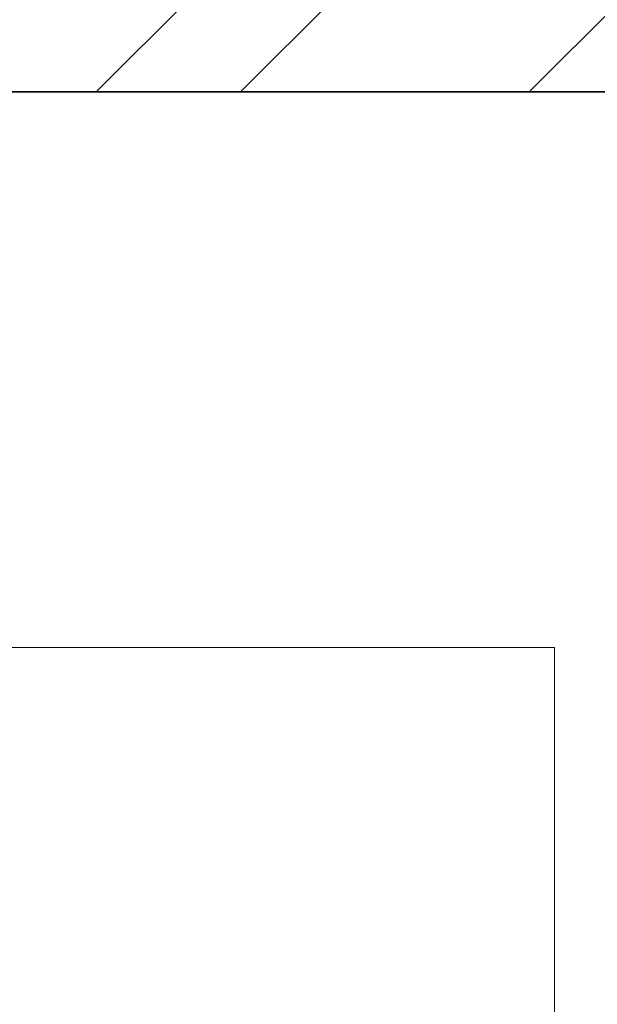
# Model space of a CAD drawing. Units: inches. Extents: x 2168 to 3056, y 1130 to 2629.
# Tile 19 of 42: x 2828 to 2846, y 2048 to 2079. Entities that reach past the tile are written whole.
import ezdxf

# ---------------------------------------------------------------- set-up
doc = ezdxf.new("R2010")
doc.units = ezdxf.units.IN
doc.layers.add('A-FLOR-CASE', color=71, linetype='Continuous', lineweight=18)
doc.layers.add('A-WALL', color=7, linetype='Continuous', lineweight=35)
doc.layers.add('A-WALL-PATT', color=143, linetype='Continuous', lineweight=13, true_color=0x7aafdf)

msp = doc.modelspace()

# ---------------------------------------------------------------- hatches: boundary and pattern name
at = {"layer": 'A-WALL-PATT'}
h = msp.add_hatch(dxfattribs=at)
h.set_pattern_fill('ANSI32', color=256)
h.paths.add_polyline_path([(2463.796, 2409.389), (2467.387, 2409.389), (2467.387, 2413.889), (2454.768, 2413.889), (2454.768, 2411.639), (2454.768, 2409.389), (2459.296, 2409.389), (2459.296, 2265.389), (2455.644, 2265.389), (2455.644, 2260.889), (2467.349, 2260.889), (2467.349, 2263.139), (2467.349, 2265.389), (2463.796, 2265.389)])
h.paths.add_polyline_path([(2431.596, 2413.889), (2409.647, 2413.889), (2409.647, 2409.389), (2431.596, 2409.389), (2431.596, 2411.639)])
h.paths.add_polyline_path([(2349.647, 2413.889), (2331.796, 2413.889), (2331.796, 2362.671), (2336.296, 2362.671), (2336.296, 2409.389), (2349.647, 2409.389), (2349.647, 2411.639)])
h.paths.add_polyline_path([(2634.149, 2411.639), (2634.149, 2413.889), (2562.293, 2413.889), (2562.293, 2409.389), (2595.796, 2409.389), (2595.796, 2280.309), (2595.826, 2280.309), (2595.826, 2265.389), (2499.91, 2265.389), (2499.91, 2260.889), (2550.796, 2260.889), (2550.796, 2117.308), (2555.296, 2117.308), (2555.296, 2168.08), (2571.93, 2168.08), (2571.93, 2176.889), (2559.796, 2176.889), (2559.796, 2256.389), (2640.796, 2256.389), (2640.796, 2176.889), (2626.428, 2176.889), (2626.428, 2168.08), (2645.296, 2168.08), (2645.296, 2116.637), (2649.796, 2116.637), (2649.796, 2260.889), (2691.251, 2260.889), (2691.251, 2263.139), (2691.251, 2265.389), (2670.655, 2265.389), (2670.655, 2265.365), (2600.296, 2265.365), (2600.296, 2280.258), (2600.296, 2409.389), (2634.149, 2409.389)])
h.paths.add_polyline_path([(2600.296, 2473.889), (2612.84, 2473.889), (2612.84, 2478.389), (2572.636, 2478.389), (2572.636, 2473.889), (2595.796, 2473.889), (2595.796, 2413.889), (2600.296, 2413.889)])
h.paths.add_polyline_path([(2535.796, 2473.889), (2548.636, 2473.889), (2548.636, 2478.389), (2531.396, 2478.389), (2531.396, 2413.889), (2521.6, 2413.889), (2521.6, 2409.389), (2539.239, 2409.389), (2539.239, 2411.639), (2539.239, 2413.889), (2535.796, 2413.889)])
h.paths.add_polyline_path([(2664.796, 2478.389), (2636.84, 2478.389), (2636.84, 2473.889), (2660.296, 2473.889), (2660.296, 2413.889), (2656.165, 2413.889), (2656.165, 2409.389), (2671.684, 2409.389), (2671.684, 2411.639), (2671.684, 2413.889), (2664.796, 2413.889)])
h.paths.add_polyline_path([(2705.942, 2413.889), (2695.684, 2413.889), (2695.684, 2409.389), (2705.942, 2409.389)])
h.paths.add_polyline_path([(2741.35, 2413.889), (2728.733, 2413.889), (2728.733, 2411.639), (2728.733, 2409.389), (2732.296, 2409.389), (2732.296, 2265.389), (2725.733, 2265.389), (2725.733, 2260.889), (2740.917, 2260.889), (2740.917, 2263.139), (2740.917, 2265.389), (2736.796, 2265.389), (2736.796, 2409.389), (2741.35, 2409.389)])
h.paths.add_polyline_path([(2785.655, 2413.889), (2764.546, 2413.889), (2764.486, 2409.389), (2785.655, 2409.389), (2785.655, 2411.639)])
h.paths.add_polyline_path([(2864.296, 2413.889), (2845.655, 2413.889), (2845.655, 2409.389), (2859.796, 2409.389), (2859.796, 2368.425), (2864.296, 2368.425)])
h.paths.add_polyline_path([(2864.296, 2308.425), (2862.046, 2308.425), (2859.796, 2308.425), (2859.796, 2265.389), (2774.483, 2265.389), (2774.483, 2263.139), (2774.483, 2260.889), (2781.796, 2260.889), (2781.796, 2226.654), (2786.296, 2226.654), (2786.296, 2260.889), (2859.796, 2260.889), (2859.796, 2241.352), (2864.296, 2241.352)])
h.paths.add_polyline_path([(2864.296, 2217.352), (2862.046, 2217.352), (2859.796, 2217.352), (2859.796, 2200.889), (2786.296, 2200.889), (2786.296, 2205.931), (2784.046, 2205.931), (2781.796, 2205.931), (2781.796, 2150.974), (2786.296, 2150.974), (2786.296, 2161.889), (2859.796, 2161.889), (2859.796, 2144.419), (2864.296, 2144.419)])
h.paths.add_polyline_path([(2859.796, 2196.389), (2859.796, 2166.389), (2786.296, 2166.389), (2786.296, 2196.389)], flags=16)
h.paths.add_polyline_path([(2864.296, 2108.419), (2862.046, 2108.419), (2859.796, 2108.419), (2859.796, 2080.889), (2786.296, 2080.889), (2786.296, 2111.993), (2781.796, 2111.993), (2781.796, 2080.889), (2649.796, 2080.889), (2649.796, 2086.036), (2647.546, 2086.036), (2645.296, 2086.036), (2645.296, 2071.739), (2649.796, 2071.739), (2649.796, 2076.389), (2781.796, 2076.389), (2781.796, 2041.792), (2786.296, 2041.792), (2786.296, 2076.389), (2859.796, 2076.389), (2859.796, 2058.577), (2864.296, 2058.577)])
h.paths.add_polyline_path([(2864.296, 2022.577), (2859.796, 2022.577), (2859.796, 1992.389), (2786.296, 1992.389), (2786.296, 1999.573), (2781.796, 1999.573), (2781.796, 1848.085), (2784.046, 1848.085), (2786.296, 1848.085), (2786.296, 1851.389), (2859.796, 1851.389), (2859.796, 1838.258), (2864.296, 1838.258)], flags=17)
h.paths.add_polyline_path([(2859.796, 1987.889), (2859.796, 1855.889), (2786.296, 1855.889), (2786.296, 1987.889)], flags=16)
h.paths.add_polyline_path([(2823.046, 1987.889), (2841.421, 1921.889), (2823.046, 1855.889)], flags=0)
h.paths.add_polyline_path([(2864.296, 1814.258), (2859.796, 1814.258), (2859.796, 1791.389), (2786.296, 1791.389), (2786.296, 1825.658), (2784.046, 1825.658), (2781.796, 1825.658), (2781.796, 1791.389), (2720.155, 1791.389), (2720.155, 1791.265), (2649.796, 1791.265), (2649.796, 1806.159), (2649.796, 2038.983), (2647.546, 2038.983), (2645.296, 2038.983), (2645.296, 1783.925), (2649.796, 1783.925), (2649.796, 1786.889), (2781.796, 1786.889), (2781.796, 1746.789), (2786.296, 1746.789), (2786.296, 1786.889), (2859.796, 1786.889), (2859.796, 1770.083), (2864.296, 1770.083)])
h.paths.add_polyline_path([(2864.296, 1734.083), (2862.046, 1734.083), (2859.796, 1734.083), (2859.796, 1705.889), (2786.296, 1705.889), (2786.296, 1714.166), (2781.796, 1714.166), (2781.796, 1660.527), (2786.296, 1660.527), (2786.296, 1666.889), (2859.796, 1666.889), (2859.796, 1648.342), (2864.296, 1648.342)])
h.paths.add_polyline_path([(2786.296, 1701.389), (2859.796, 1701.389), (2859.796, 1671.389), (2786.296, 1671.389)], flags=16)
h.paths.add_polyline_path([(2649.796, 1756.576), (2647.546, 1756.576), (2645.296, 1756.576), (2645.296, 1606.889), (2555.296, 1606.889), (2555.296, 1749.513), (2553.046, 1749.513), (2550.796, 1749.513), (2550.796, 1606.889), (2503.006, 1606.889), (2503.006, 1604.639), (2503.006, 1602.389), (2595.796, 1602.389), (2595.849, 1602.389), (2595.849, 1587.495), (2595.796, 1458.389), (2561.502, 1458.389), (2561.502, 1456.139), (2561.502, 1453.889), (2595.796, 1453.889), (2595.796, 1381.889), (2573.438, 1381.889), (2573.438, 1377.389), (2613.01, 1377.389), (2613.01, 1379.639), (2613.01, 1381.889), (2600.296, 1381.889), (2600.296, 1453.889), (2634.327, 1453.889), (2634.327, 1458.389), (2600.296, 1458.389), (2600.296, 1602.389), (2670.655, 1602.389), (2694.095, 1602.389), (2694.095, 1606.889), (2649.796, 1606.889)])
h.paths.add_polyline_path([(2736.796, 1602.389), (2741.562, 1602.389), (2741.562, 1606.889), (2726.203, 1606.889), (2726.203, 1604.639), (2726.203, 1602.389), (2732.296, 1602.389), (2732.296, 1458.389), (2727.899, 1458.389), (2727.899, 1453.889), (2740.821, 1453.889), (2740.821, 1456.139), (2740.821, 1458.389), (2736.796, 1458.389)])
h.paths.add_polyline_path([(2859.796, 1606.889), (2786.296, 1606.889), (2786.296, 1637.334), (2784.046, 1637.334), (2781.796, 1637.334), (2781.796, 1606.889), (2775.612, 1606.889), (2775.612, 1602.389), (2859.796, 1602.389)])
h.paths.add_polyline_path([(2864.296, 1624.342), (2862.046, 1624.342), (2859.796, 1624.342), (2859.796, 1570.39), (2864.296, 1570.39)])
h.paths.add_polyline_path([(2864.296, 1510.39), (2862.046, 1510.39), (2859.796, 1510.39), (2859.796, 1458.389), (2846.735, 1458.389), (2846.735, 1456.139), (2846.735, 1453.889), (2864.296, 1453.889)])
h.paths.add_polyline_path([(2786.735, 1458.389), (2765.444, 1458.389), (2765.444, 1453.889), (2786.735, 1453.889)])
h.paths.add_polyline_path([(2706.004, 1458.389), (2695.36, 1458.389), (2695.36, 1453.889), (2706.004, 1453.889), (2706.004, 1456.139)])
h.paths.add_polyline_path([(2671.36, 1456.139), (2671.36, 1458.389), (2655.986, 1458.389), (2655.986, 1456.139), (2655.986, 1453.889), (2660.296, 1453.889), (2660.296, 1381.889), (2637.01, 1381.889), (2637.01, 1377.389), (2664.796, 1377.389), (2664.796, 1453.889), (2671.36, 1453.889)], flags=17)
h.paths.add_polyline_path([(2539.829, 1458.389), (2520.237, 1458.389), (2520.237, 1453.889), (2531.296, 1453.889), (2531.296, 1377.389), (2546.449, 1377.389), (2546.449, 1379.639), (2546.449, 1381.889), (2535.796, 1381.889), (2535.796, 1453.889), (2539.829, 1453.889)], flags=17)
h.paths.add_polyline_path([(2496.237, 1458.389), (2489.13, 1458.389), (2489.13, 1453.889), (2496.237, 1453.889), (2496.237, 1456.139)])
h.paths.add_polyline_path([(2467.433, 1456.139), (2467.433, 1458.389), (2463.796, 1458.389), (2463.796, 1602.389), (2468.242, 1602.389), (2468.242, 1605.7), (2468.242, 1606.889), (2454.602, 1606.889), (2454.602, 1602.389), (2459.296, 1602.389), (2459.296, 1458.389), (2454.24, 1458.389), (2454.24, 1453.889), (2467.433, 1453.889)])
h.paths.add_polyline_path([(2431.601, 1456.139), (2431.601, 1458.389), (2411.386, 1458.389), (2411.386, 1453.889), (2431.601, 1453.889)])
h.paths.add_polyline_path([(2351.386, 1458.389), (2336.296, 1458.389), (2336.296, 1490.693), (2334.046, 1490.693), (2331.796, 1490.693), (2331.796, 1453.889), (2351.386, 1453.889), (2351.386, 1456.139)])
h.paths.add_polyline_path([(2336.296, 1629.705), (2331.796, 1629.705), (2331.796, 1552.317), (2336.296, 1552.317), (2336.296, 1602.389), (2406.655, 1602.389), (2423.472, 1602.389), (2423.472, 1606.889), (2418.796, 1606.889), (2418.796, 1643.678), (2416.546, 1643.678), (2414.296, 1643.678), (2414.296, 1606.889), (2336.296, 1606.889)])
h.paths.add_polyline_path([(2418.796, 1714.384), (2414.296, 1714.384), (2414.296, 1705.889), (2336.296, 1705.889), (2336.296, 1731.324), (2334.046, 1731.324), (2331.796, 1731.324), (2331.796, 1653.705), (2334.046, 1653.705), (2336.296, 1653.705), (2336.296, 1666.889), (2414.296, 1666.889), (2414.296, 1663.589), (2418.796, 1663.589)])
h.paths.add_polyline_path([(2336.296, 1701.389), (2414.296, 1701.389), (2414.296, 1671.389), (2336.296, 1671.389)], flags=16)
h.paths.add_polyline_path([(2555.296, 2040.059), (2550.796, 2040.059), (2550.796, 1791.389), (2550.561, 1791.205), (2480.202, 1791.205), (2418.796, 1791.389), (2418.796, 1825.448), (2416.546, 1825.448), (2414.296, 1825.448), (2414.296, 1791.389), (2336.296, 1791.389), (2336.296, 1806.409), (2331.796, 1806.409), (2331.796, 1767.324), (2336.296, 1767.324), (2336.296, 1786.889), (2414.296, 1786.889), (2414.296, 1745.457), (2418.796, 1745.457), (2418.796, 1786.889), (2550.796, 1786.889), (2550.796, 1783.011), (2555.296, 1783.011)])
h.paths.add_polyline_path([(2418.796, 1923.389), (2423.207, 1923.389), (2423.207, 1925.639), (2423.207, 1927.889), (2418.796, 1927.889), (2418.796, 2000.048), (2414.296, 2000.048), (2414.296, 1992.389), (2336.296, 1992.389), (2336.296, 1987.889), (2414.296, 1987.889), (2414.296, 1855.889), (2336.296, 1855.889), (2336.296, 1851.389), (2414.296, 1851.389), (2414.296, 1846.759), (2418.796, 1846.759)], flags=17)
h.paths.add_polyline_path([(2336.296, 2019.294), (2334.046, 2019.294), (2331.796, 2019.294), (2331.796, 1830.409), (2336.296, 1830.409)], flags=17)
h.paths.add_polyline_path([(2550.796, 1927.889), (2453.541, 1927.889), (2453.541, 1925.639), (2453.541, 1923.389), (2550.796, 1923.389)], flags=17)
h.paths.add_polyline_path([(2744.987, 1927.889), (2649.796, 1927.889), (2649.796, 1923.389), (2744.987, 1923.389), (2744.987, 1925.639)], flags=17)
h.paths.add_polyline_path([(2555.296, 2086.458), (2553.046, 2086.458), (2550.796, 2086.458), (2550.796, 2080.889), (2418.796, 2080.889), (2336.296, 2080.889), (2336.296, 2115.399), (2334.046, 2115.399), (2331.796, 2115.399), (2331.796, 2055.294), (2336.296, 2055.294), (2336.296, 2076.389), (2550.796, 2076.389), (2550.796, 2071.538), (2555.296, 2071.538)])
h.paths.add_polyline_path([(2418.796, 2121.389), (2414.296, 2121.389), (2414.296, 2080.889), (2418.796, 2080.889)])
h.paths.add_polyline_path([(2418.796, 2076.389), (2414.296, 2076.389), (2414.296, 2035.123), (2418.796, 2035.123)])
h.paths.add_polyline_path([(2422.868, 2263.139), (2422.868, 2265.389), (2406.655, 2265.389), (2406.655, 2265.359), (2336.296, 2265.359), (2336.296, 2280.252), (2336.296, 2302.671), (2334.046, 2302.671), (2331.796, 2302.671), (2331.796, 2246.853), (2336.296, 2246.853), (2336.296, 2260.889), (2414.296, 2260.889), (2414.296, 2223.996), (2418.796, 2223.996), (2418.796, 2260.889), (2422.868, 2260.889)])
h.paths.add_polyline_path([(2418.796, 2204.783), (2416.546, 2204.783), (2414.296, 2204.783), (2414.296, 2200.889), (2336.296, 2200.889), (2336.296, 2220.853), (2331.796, 2220.853), (2331.796, 2151.399), (2336.296, 2151.399), (2336.296, 2161.889), (2414.296, 2161.889), (2414.296, 2153.726), (2418.796, 2153.726)])
h.paths.add_polyline_path([(2414.296, 2196.389), (2414.296, 2166.389), (2336.296, 2166.389), (2336.296, 2196.389)], flags=16)
h.paths.add_polyline_path([(2375.296, 2181.389), (2336.296, 2166.389), (2336.296, 2196.389)], flags=0)
h.paths.add_polyline_path([(2809.595, 2172.34), (2838.804, 2172.34), (2838.804, 2190.997), (2809.595, 2190.997)], flags=8)
h.paths.add_polyline_path([(2849.75, 1919.585), (2849.75, 1952.672), (2831.093, 1952.672), (2831.093, 1919.585)], flags=8)
h.paths.add_polyline_path([(2808.875, 1901.967), (2808.875, 1937.85), (2790.149, 1937.85), (2790.149, 1901.967)], flags=8)
h.paths.add_polyline_path([(2806.285, 1671.896), (2835.493, 1671.896), (2835.493, 1690.553), (2806.285, 1690.553)], flags=8)
h.paths.add_polyline_path([(2353.186, 1676.549), (2382.395, 1676.549), (2382.395, 1695.207), (2353.186, 1695.207)], flags=8)
h.paths.add_polyline_path([(2360.083, 1832.308), (2389.241, 1832.308), (2389.241, 1850.966), (2360.083, 1850.966)], flags=25)
h.paths.add_polyline_path([(2354.822, 2167.823), (2384.031, 2167.823), (2384.031, 2186.481), (2354.822, 2186.481)], flags=8)

# ---------------------------------------------------------------- linework, layer by layer
at = {"layer": 'A-FLOR-CASE'}
for p, q in [((2786.296, 2059.09), (2844.993, 2059.09)), ((2844.993, 2059.09), (2844.993, 1992.389))]:
    msp.add_line(p, q, dxfattribs=at)
at = {"layer": 'A-WALL'}
msp.add_line((2786.296, 2076.389), (2859.796, 2076.389), dxfattribs=at)

doc.saveas('drawing.dxf')
